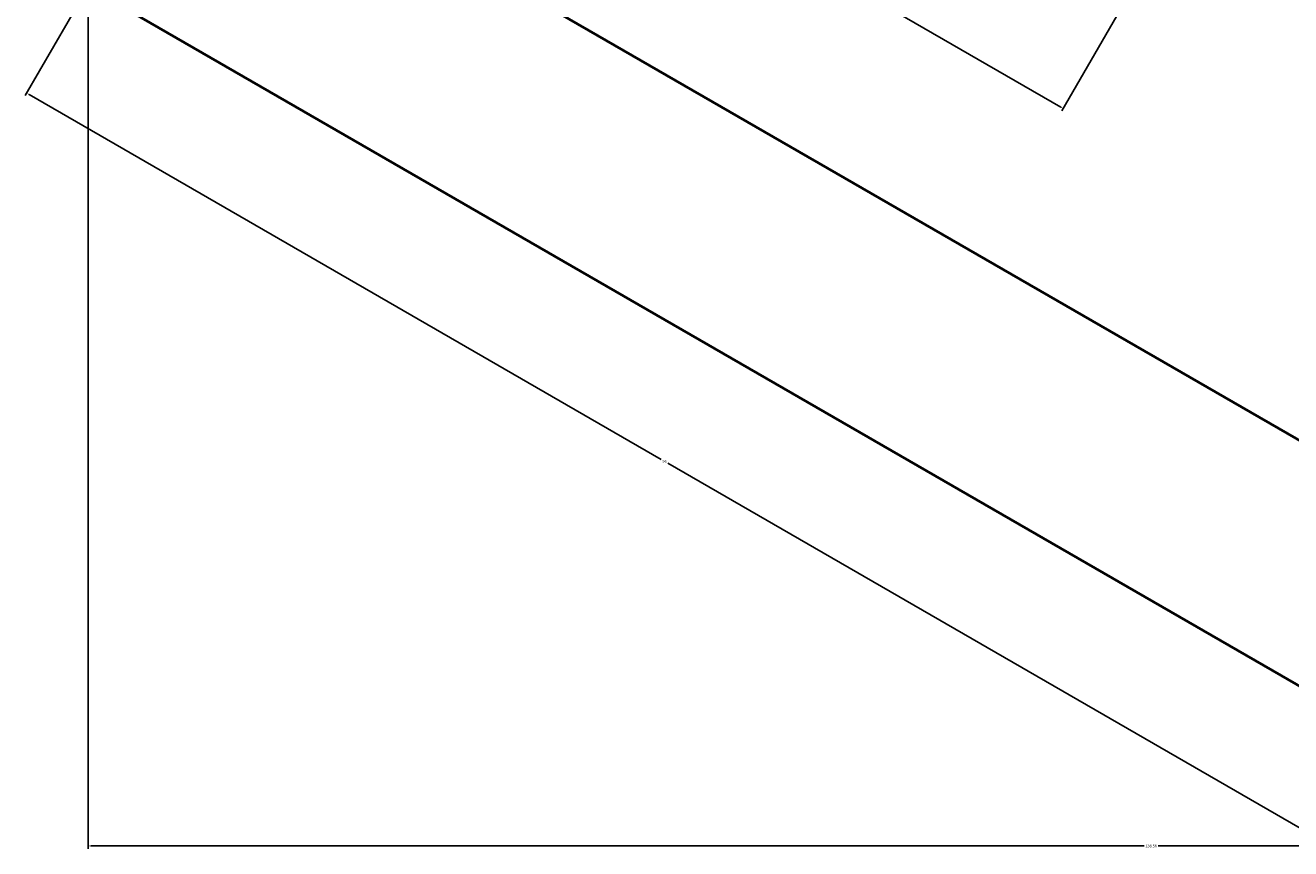
# Model space of a CAD drawing. Units: millimetres. Extents: x 2919 to 3075, y 2801 to 2951.
# Tile 1 of 14: x 2924 to 3006, y 2801 to 2854. Entities that reach past the tile are written whole.
import ezdxf

# ---------------------------------------------------------------- set-up
doc = ezdxf.new("R2010")
doc.units = ezdxf.units.MM
doc.layers.add('M-DIMS', color=2, linetype='Continuous', lineweight=18)
doc.layers.add('M-OUTL', color=7, linetype='Continuous', lineweight=50)
doc.styles.get("Standard").update_dxf_attribs({"font": 'arial.ttf'})
doc.dimstyles.get("Standard").update_dxf_attribs({"dimtxt": 0.18, "dimasz": 0.18, "dimexe": 0.18, "dimexo": 0.0625, "dimgap": 0.09, "dimtad": 0, "dimtih": 1, "dimtoh": 1, "dimdec": 4, "dimzin": 0, "dimdsep": 46, "dimtxsty": 'Standard', "dimcen": 0.09, "dimadec": 0, "dimazin": 0, "dimtfac": 1, "dimtdec": 4, "dimtofl": 0, "dimtmove": 0, "dimatfit": 3, "dimfxl": 1, "dimtolj": 1, "dimtzin": 0, "dimarcsym": 0})

# ---------------------------------------------------------------- blocks, each defined once
blk = doc.blocks.new('*D1')
at = {"layer": 'Defpoints', "color": 0, "transparency": 16777216}
for p in [(2987.323, 2944.203), (3074.337, 2944.203), (3010.912, 2808.893)]:
    blk.add_point(p, dxfattribs=at)
at = {"layer": 'M-DIMS', "color": 0, "lineweight": -2, "transparency": 16777216}
for p, q in [((2987.386, 2944.203), (3074.517, 2944.203)), ((3074.337, 2944.023), (3074.337, 2876.73)), ((3074.337, 2809.073), (3074.337, 2876.366)), ((3010.974, 2808.893), (3074.517, 2808.893))]:
    blk.add_line(p, q, dxfattribs=at)
at = {"layer": 'M-DIMS', "color": 0, "transparency": 16777216}
for points in [[(3074.307, 2944.023), (3074.367, 2944.023), (3074.337, 2944.203)], [(3074.307, 2809.073), (3074.367, 2809.073), (3074.337, 2808.893)]]:
    blk.add_solid(points, dxfattribs=at)
at = {"layer": 'M-DIMS', "color": 0, "transparency": 16777216, "insert": (3074.337, 2876.548), "char_height": 0.18, "attachment_point": 5}
blk.add_mtext('\\A1;135.3', dxfattribs=at)
blk = doc.blocks.new('*D2')
at = {"layer": 'Defpoints', "color": 0, "transparency": 16777216}
for p in [(2927.773, 2856.893), (3066.337, 2840.893), (3066.337, 2800.893)]:
    blk.add_point(p, dxfattribs=at)
at = {"layer": 'M-DIMS', "color": 0, "lineweight": -2, "transparency": 16777216}
for p, q in [((2927.773, 2856.831), (2927.773, 2800.713)), ((3066.337, 2840.831), (3066.337, 2800.713)), ((2927.953, 2800.893), (2996.6, 2800.893)), ((3066.157, 2800.893), (2997.51, 2800.893))]:
    blk.add_line(p, q, dxfattribs=at)
at = {"layer": 'M-DIMS', "color": 0, "transparency": 16777216}
for points in [[(2927.953, 2800.923), (2927.953, 2800.863), (2927.773, 2800.893)], [(3066.157, 2800.923), (3066.157, 2800.863), (3066.337, 2800.893)]]:
    blk.add_solid(points, dxfattribs=at)
at = {"layer": 'M-DIMS', "color": 0, "transparency": 16777216, "insert": (2997.055, 2800.893), "char_height": 0.18, "attachment_point": 5}
blk.add_mtext('\\A1;138.56', dxfattribs=at)
blk = doc.blocks.new('*D3')
at = {"layer": 'Defpoints', "color": 0, "transparency": 16777216}
for p in [(2927.773, 2856.893), (2923.773, 2849.965), (3010.912, 2808.893)]:
    blk.add_point(p, dxfattribs=at)
at = {"layer": 'M-DIMS', "color": 0, "lineweight": -2, "transparency": 16777216}
for p, q in [((2927.742, 2856.839), (2923.683, 2849.809)), ((2923.929, 2849.875), (2965.124, 2826.091)), ((3006.756, 2802.055), (2965.561, 2825.839)), ((3010.88, 2808.839), (3006.822, 2801.809))]:
    blk.add_line(p, q, dxfattribs=at)
at = {"layer": 'M-DIMS', "color": 0, "transparency": 16777216}
for points in [[(2923.944, 2849.901), (2923.914, 2849.849), (2923.773, 2849.965)], [(3006.771, 2802.081), (3006.741, 2802.029), (3006.912, 2801.965)]]:
    blk.add_solid(points, dxfattribs=at)
at = {"layer": 'M-DIMS', "color": 0, "transparency": 16777216, "insert": (2965.342, 2825.965), "char_height": 0.18, "attachment_point": 5}
blk.add_mtext('\\A1;96', dxfattribs=at)
blk = doc.blocks.new('*D11')
at = {"layer": 'Defpoints', "color": 0, "transparency": 16777216}
for p in [(2960.682, 2875.893), (2956.682, 2868.965), (2995.323, 2855.893)]:
    blk.add_point(p, dxfattribs=at)
at = {"layer": 'M-DIMS', "color": 0, "lineweight": -2, "transparency": 16777216}
for p, q in [((2960.651, 2875.839), (2956.592, 2868.809)), ((2956.838, 2868.875), (2973.78, 2859.093)), ((2991.167, 2849.055), (2974.225, 2858.837)), ((2995.292, 2855.839), (2991.233, 2848.809))]:
    blk.add_line(p, q, dxfattribs=at)
at = {"layer": 'M-DIMS', "color": 0, "transparency": 16777216}
for points in [[(2956.853, 2868.901), (2956.823, 2868.849), (2956.682, 2868.965)], [(2991.182, 2849.081), (2991.152, 2849.029), (2991.323, 2848.965)]]:
    blk.add_solid(points, dxfattribs=at)
at = {"layer": 'M-DIMS', "color": 0, "transparency": 16777216, "insert": (2974.003, 2858.965), "char_height": 0.18, "attachment_point": 5}
blk.add_mtext('\\A1;40', dxfattribs=at)

msp = doc.modelspace()

# ---------------------------------------------------------------- linework, layer by layer
at = {"layer": 'M-OUTL'}
for p, q in [((3010.9116, 2824.8932), (2941.6296, 2864.8932)), ((2927.7732, 2856.8932), (3010.9116, 2808.8932))]:
    msp.add_line(p, q, dxfattribs=at)

# ---------------------------------------------------------------- dimensions: what is measured, and where the dimension line sits
at = {"layer": 'M-DIMS'}
for base, p1, p2, angle, override, picture, middle in [((3074.3372, 2944.2026), (3010.9116, 2808.8932), (2987.3232, 2944.2026), 90, {"dimdec": 1, "dimlfac": 1, "dimrnd": 0, "dimzin": 0, "dimdsep": 46, "dimlunit": 2}, '*D1', (3074.3372, 2876.5479)), ((2956.6821, 2868.965), (2995.3232, 2855.8932), (2960.6821, 2875.8932), 150, {"dimdec": 0, "dimlfac": 1, "dimrnd": 0, "dimzin": 0, "dimdsep": 46, "dimlunit": 2}, '*D11', (2974.0027, 2858.965)), ((2923.7732, 2849.965), (3010.9116, 2808.8932), (2927.7732, 2856.8932), 150, {"dimdec": 0, "dimlfac": 1, "dimrnd": 0, "dimzin": 0, "dimdsep": 46, "dimlunit": 2}, '*D3', (2965.3424, 2825.965))]:
    dim = msp.add_linear_dim(base=base, p1=p1, p2=p2, angle=angle, dimstyle='Standard', override=override, dxfattribs=at)
    dim.commit()
    dim.dimension.update_dxf_attribs({"geometry": picture, "text_midpoint": middle})
dim = msp.add_linear_dim(base=(3066.3372, 2800.8932), p1=(2927.7732, 2856.8932), p2=(3066.3372, 2840.8932), dimstyle='Standard', override={"dimdec": 2, "dimlfac": 1, "dimrnd": 0, "dimzin": 0, "dimdsep": 46, "dimlunit": 2}, dxfattribs=at)
dim.commit()
dim.dimension.update_dxf_attribs({"geometry": '*D2', "text_midpoint": (2997.0552, 2800.8932)})

doc.saveas('drawing.dxf')
